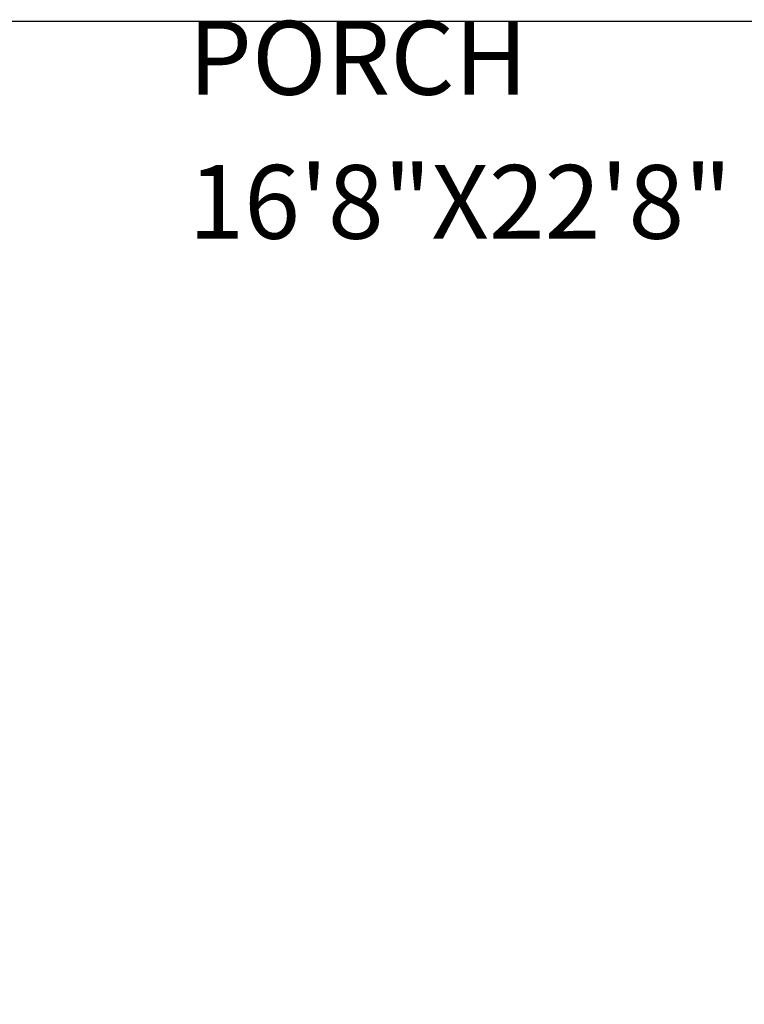
# Model space of a CAD drawing. Units: inches. Extents: x 1319 to 2030, y 219 to 1069.
# Tile 15 of 28: x 1506 to 1565, y 392 to 472. Entities that reach past the tile are written whole.
import ezdxf

# ---------------------------------------------------------------- set-up
doc = ezdxf.new("R2010")
doc.units = ezdxf.units.IN
doc.header["$MEASUREMENT"] = 0
doc.layers.add('A-ANNO-DIMS', color=2, linetype='Continuous', lineweight=18)
doc.layers.add('A-AREA-IDEN', color=250, linetype='Continuous', lineweight=18)
doc.styles.get("Standard").update_dxf_attribs({"font": 'arial.ttf'})
doc.dimstyles.get("Standard").update_dxf_attribs({"dimtxt": 7, "dimasz": 0.18, "dimexe": 0.18, "dimexo": 0.0625, "dimgap": 0.09, "dimtad": 0, "dimtih": 1, "dimtoh": 1, "dimzin": 0, "dimdsep": 46, "dimlunit": 3, "dimtxsty": 'Standard', "dimcen": 0.09, "dimadec": 0, "dimazin": 0, "dimtfac": 1, "dimtofl": 0, "dimtmove": 0, "dimatfit": 3, "dimfxl": 1, "dimtolj": 1, "dimtzin": 0, "dimarcsym": 0})

# ---------------------------------------------------------------- blocks, each defined once
blk = doc.blocks.new('*D65')
at = {"layer": 'A-ANNO-DIMS', "color": 0, "lineweight": -2, "transparency": 16777216}
for p, q in [((1648.280254, 472.227245), (1329.112754, 472.227245)), ((1329.292754, 472.047245), (1329.292754, 431.817245)), ((1329.292754, 384.407245), (1329.292754, 424.637245)), ((1648.280254, 384.227245), (1329.112754, 384.227245))]:
    blk.add_line(p, q, dxfattribs=at)
at = {"layer": 'A-ANNO-DIMS', "color": 0, "transparency": 16777216}
for points in [[(1329.262754, 472.047245), (1329.322754, 472.047245), (1329.292754, 472.227245)], [(1329.262754, 384.407245), (1329.322754, 384.407245), (1329.292754, 384.227245)]]:
    blk.add_solid(points, dxfattribs=at)
at = {"layer": 'Defpoints', "color": 0, "transparency": 16777216}
for p in [(1329.292754, 472.227245), (1648.342754, 472.227245), (1648.342754, 384.227245)]:
    blk.add_point(p, dxfattribs=at)
at = {"layer": 'A-ANNO-DIMS', "color": 0, "transparency": 16777216, "insert": (1329.292754, 428.227245), "char_height": 7, "attachment_point": 5}
blk.add_mtext('\\A1;7\'-4"', dxfattribs=at)

msp = doc.modelspace()

# ---------------------------------------------------------------- texts
at = {"layer": 'A-AREA-IDEN'}
for s, height, p in [('PORCH', 6.0112, (1519.684, 466.259)), ('16\'8"X22\'8"', 6.01124, (1519.684, 454.51))]:
    msp.add_text(s, height=height, dxfattribs=at).set_placement(p)

# ---------------------------------------------------------------- dimensions: what is measured, and where the dimension line sits
at = {"layer": 'A-ANNO-DIMS'}
dim = msp.add_linear_dim(base=(1329.293, 472.227), p1=(1648.343, 384.227), p2=(1648.343, 472.227), angle=90, dimstyle='Standard', override={"dimdec": 1, "dimlfac": 1, "dimrnd": 0, "dimzin": 1, "dimdsep": 46, "dimlunit": 4, "dimfrac": 2}, dxfattribs=at)
dim.commit()
dim.dimension.update_dxf_attribs({"geometry": '*D65', "text_midpoint": (1329.293, 428.227)})

doc.saveas('drawing.dxf')
